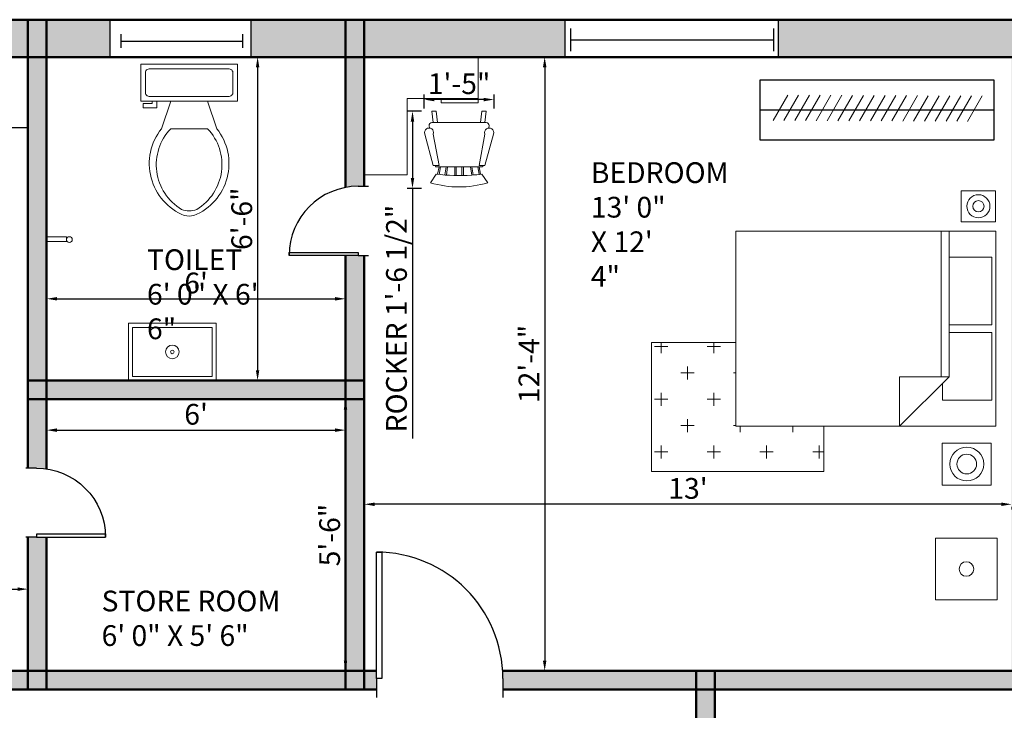
# Model space of a CAD drawing. Units: millimetres. Extents: x 3107 to 3757, y 777 to 1464.
# Tile 6 of 7: x 3301 to 3539, y 1284 to 1450. Entities that reach past the tile are written whole.
import ezdxf

# ---------------------------------------------------------------- set-up
doc = ezdxf.new("R2010")
doc.units = ezdxf.units.MM
for name, color, linetype, lineweight in [('A-ANNO-DIMS', 50, 'Continuous', 18), ('A-AREA-IDEN', 160, 'Continuous', 18), ('A-FLOR-CASE', 140, 'Continuous', 25), ('A-FLOR-CASE-PATT', 140, 'Continuous', 13), ('A-FLOR-FIXT', 140, 'Continuous', 18), ('A-FURN-PATT', 140, 'Continuous', 13), ('A-WALL-PATT', 80, 'Continuous', 13), ('doors', 10, 'Continuous', 25), ('furniture', 140, 'Continuous', 18), ('walls', 80, 'Continuous', 50), ('windows', 30, 'Continuous', 25)]:
    doc.layers.add(name, color=color, linetype=linetype, lineweight=lineweight)
doc.styles.get("Standard").update_dxf_attribs({"font": 'arial.ttf'})
doc.dimstyles.new('ISO-25', dxfattribs={"dimtxt": 5, "dimasz": 2.5, "dimexe": 1.25, "dimexo": 0.625, "dimtad": 1, "dimdec": 0, "dimlunit": 3, "dimtxsty": 'Standard', "dimcen": 2.5, "dimadec": 0, "dimazin": 0, "dimtfac": 1, "dimtdec": 0, "dimtmove": 0, "dimatfit": 3, "dimfxl": 1, "dimarcsym": 0})

# ---------------------------------------------------------------- blocks, each defined once
blk = doc.blocks.new('*U2')
for p, q in [((0, 0), (0, -6)), ((40, 0), (40, -6))]:
    blk.add_line(p, q)
blk.add_lwpolyline([(0, 0), (0, 40), (1.75, 40), (1.75, 0)], close=True)
blk.add_arc((0, 0), 40, 0, 90)
blk = doc.blocks.new('*U5')
for p, q in [((0, 4), (0, 0)), ((36, 4), (36, 0)), ((0, 2), (36, 2))]:
    blk.add_line(p, q)
blk = doc.blocks.new('*U4')
for p, q in [((0, 4), (0, 0)), ((36, 4), (36, 0)), ((0, 2), (36, 2))]:
    blk.add_line(p, q)
blk = doc.blocks.new('Toilet - top')
for p, q in [((9.5, -6), (9.5, -2)), ((-10, -8.5), (-8, -8.5)), ((-10, -9.5), (-10, -8.5)), ((-8, -8.5), (-8, -8)), ((-7, -8), (-7, -9.5)), ((-4, -8), (-6, -14)), ((4, -8), (6, -14)), ((-7, -9.5), (-10, -9.5)), ((4, -14), (-4, -14))]:
    blk.add_line(p, q)
blk.add_lwpolyline([(10.5, -8), (10.5, 0), (-10.5, 0), (-10.5, -8)], close=True)
for points in [[(-9.5, -2), (-9.5, -6)], [(8.5, -1), (-8.5, -1)], [(-8.5, -7), (8.5, -7)]]:
    blk.add_lwpolyline(points)
for centre, radius, start, end in [((-8.62, -1.88), 0.884, 81.8699, 188.1301), ((8.62, -1.88), 0.884, 351.8699, 98.1301), ((-8.62, -6.12), 0.884, 171.8699, 278.1301), ((8.62, -6.12), 0.884, 261.8699, 8.1301), ((3.52, -21.58), 12.17, 141.4691, 247.9714), ((4.2, -21.82), 11.33, 136.3677, 238.9468), ((-3.52, -21.58), 12.17, 292.0284, 38.5307), ((-4.2, -21.82), 11.33, 301.053, 43.6321), ((0, -27.88), 4, 245.7318, 294.2682), ((0, -29), 4, 254.8605, 285.1395)]:
    blk.add_arc(centre, radius, start, end)
blk = doc.blocks.new('Chair - Rocking')
for p, q in [((-8, -4.5), (-10, -1.5)), ((8, -4.5), (10, -1.5)), ((-7.5, -4.5), (-7, -7)), ((-6.5, -7), (-7.02225, -4.43)), ((-4.5, -7), (-4.96674, -4.19951)), ((-4, -7), (-4.40532, -4.16272)), ((-1.5, -4.05012), (-1.5, -7)), ((-1, -7), (-1, -4.05012)), ((1, -7), (1, -4.04655)), ((1.5, -4.05012), (1.5, -7)), ((4, -7), (4.40187, -4.18694)), ((4.5, -7), (4.96761, -4.19437)), ((6.5, -7), (7, -4.4057)), ((7.5, -4.5), (7, -7)), ((-9, -7.5), (-12, -18.49999)), ((-7, -7.5), (-9, -7.5)), ((-9, -18.49999), (-7, -7.5)), ((-8.23428, -6.99939), (-8.3093, -7.47958)), ((-8.23041, -7), (8.23915, -7)), ((7, -7.5), (9, -7.5)), ((9, -18.49999), (7, -7.5)), ((8.31071, -7.48854), (8.23449, -7.00073)), ((9, -7.5), (12, -18.49999)), ((10.5, -21.49999), (10.3575, -20.58798)), ((-10.36644, -20.64523), (-10.5, -21.49999)), ((-9, -22.49999), (-9.5, -26.49999)), ((0, -22.49999), (-9.5, -22.49999)), ((-8, -26.49999), (-7.5, -22.49999)), ((0, -22.49999), (9.5, -22.49999)), ((8, -26.49999), (7.5, -22.49999)), ((9, -22.49999), (9.5, -26.49999)), ((-9.5, -26.49999), (-8, -26.49999)), ((9.5, -26.49999), (8, -26.49999))]:
    blk.add_line(p, q)
for centre, radius, start, end in [((0, -34.08333), 34.08333, 72.93847, 107.0615), ((0, -68.25004), 64.25, 93.92211, 97.15267), ((0, -68.25004), 64.25, 82.84733, 93.92211), ((-10.5, -18.99999), 1.58114, 161.5651, 18.43495), ((10.5, -18.99999), 1.58114, 161.5651, 18.43495), ((-9.5, -21.49999), 1, 180, 270), ((9.5, -21.49999), 1, 270, 0)]:
    blk.add_arc(centre, radius, start, end)
blk = doc.blocks.new('Bed - Queen')
for p, q in [((0, -80.00003), (0, 0)), ((0, 0), (59.99999, 0)), ((59.99999, 0), (59.99999, -80.00003)), ((7.99999, -1.2), (28.79998, -1.2)), ((7.99999, -14.4), (7.99999, -1.2)), ((28.79998, -1.2), (28.79998, -14.4)), ((31.19999, -1.2), (51.99999, -1.2)), ((31.19999, -14.4), (31.19999, -1.2)), ((51.99999, -1.2), (51.99999, -16.4)), ((0, -14.4), (44.8, -14.4)), ((59.99999, -29.6), (44.8, -14.4)), ((44.8, -14.4), (44.8, -29.6)), ((44.8, -16.8), (0, -16.8)), ((51.99999, -16.4), (46.79936, -16.4)), ((44.8, -29.6), (59.99999, -29.6)), ((59.99999, -80.00003), (0, -80.00003))]:
    blk.add_line(p, q)
blk = doc.blocks.new('*D17')
at = {"layer": 'A-ANNO-DIMS', "color": 0, "lineweight": -2, "transparency": 16777216}
for p, q in [((3119.47, 1311.37), (3119.47, 1314.39)), ((3121.97, 1313.14), (3300.97, 1313.14)), ((3303.47, 1313.51), (3303.47, 1311.89))]:
    blk.add_line(p, q, dxfattribs=at)
at = {"layer": 'A-ANNO-DIMS', "color": 0, "transparency": 16777216}
for points in [[(3121.97, 1313.56), (3121.97, 1312.72), (3119.47, 1313.14)], [(3300.97, 1313.56), (3300.97, 1312.72), (3303.47, 1313.14)]]:
    blk.add_solid(points, dxfattribs=at)
at = {"layer": 'Defpoints', "color": 0, "transparency": 16777216}
for p in [(3303.47, 1314.14), (3303.47, 1313.14), (3119.47, 1310.75)]:
    blk.add_point(p, dxfattribs=at)
at = {"layer": 'A-ANNO-DIMS', "color": 0, "transparency": 16777216, "insert": (3211.47, 1316.32), "char_height": 5, "attachment_point": 5}
blk.add_mtext('15\'-4"', dxfattribs=at)
blk = doc.blocks.new('*D18')
at = {"layer": 'A-ANNO-DIMS', "color": 0, "lineweight": -2, "transparency": 16777216}
for p, q in [((3358.24, 1441.43), (3357.54, 1441.43)), ((3358.79, 1438.93), (3358.79, 1365.93)), ((3358.24, 1363.43), (3357.54, 1363.43))]:
    blk.add_line(p, q, dxfattribs=at)
at = {"layer": 'A-ANNO-DIMS', "color": 0, "transparency": 16777216}
for points in [[(3358.38, 1438.93), (3359.21, 1438.93), (3358.79, 1441.43)], [(3358.38, 1365.93), (3359.21, 1365.93), (3358.79, 1363.43)]]:
    blk.add_solid(points, dxfattribs=at)
at = {"layer": 'Defpoints', "color": 0, "transparency": 16777216}
for p in [(3358.87, 1441.43), (3358.79, 1363.43), (3358.87, 1363.43)]:
    blk.add_point(p, dxfattribs=at)
at = {"layer": 'A-ANNO-DIMS', "color": 0, "transparency": 16777216, "insert": (3355.62, 1402.43), "char_height": 5, "attachment_point": 5, "rotation": 90}
blk.add_mtext('6\'-6"', dxfattribs=at)
blk = doc.blocks.new('*D19')
at = {"layer": 'A-ANNO-DIMS', "color": 0, "lineweight": -2, "transparency": 16777216}
for p, q in [((3307.97, 1383.76), (3307.97, 1384.39)), ((3310.47, 1383.14), (3377.47, 1383.14)), ((3379.97, 1383.76), (3379.97, 1384.39))]:
    blk.add_line(p, q, dxfattribs=at)
at = {"layer": 'A-ANNO-DIMS', "color": 0, "transparency": 16777216}
for points in [[(3310.47, 1383.55), (3310.47, 1382.72), (3307.97, 1383.14)], [(3377.47, 1383.55), (3377.47, 1382.72), (3379.97, 1383.14)]]:
    blk.add_solid(points, dxfattribs=at)
at = {"layer": 'Defpoints', "color": 0, "transparency": 16777216}
for p in [(3307.97, 1383.14), (3379.97, 1383.14), (3379.97, 1383.14)]:
    blk.add_point(p, dxfattribs=at)
at = {"layer": 'A-ANNO-DIMS', "color": 0, "transparency": 16777216, "insert": (3343.97, 1386.31), "char_height": 5, "attachment_point": 5}
blk.add_mtext("6'", dxfattribs=at)
blk = doc.blocks.new('*D20')
at = {"layer": 'A-ANNO-DIMS', "color": 0, "lineweight": -2, "transparency": 16777216}
for p, q in [((3384.47, 1334.22), (3384.47, 1334.85)), ((3537.97, 1333.6), (3386.97, 1333.6)), ((3540.47, 1332.97), (3540.47, 1332.35))]:
    blk.add_line(p, q, dxfattribs=at)
at = {"layer": 'A-ANNO-DIMS', "color": 0, "transparency": 16777216}
for points in [[(3386.97, 1334.01), (3386.97, 1333.18), (3384.47, 1333.6)], [(3537.97, 1334.01), (3537.97, 1333.18), (3540.47, 1333.6)]]:
    blk.add_solid(points, dxfattribs=at)
at = {"layer": 'Defpoints', "color": 0, "transparency": 16777216}
for p in [(3384.47, 1333.6), (3384.47, 1333.6), (3540.47, 1333.6)]:
    blk.add_point(p, dxfattribs=at)
at = {"layer": 'A-ANNO-DIMS', "color": 0, "transparency": 16777216, "insert": (3462.47, 1336.78), "char_height": 5, "attachment_point": 5}
blk.add_mtext("13'", dxfattribs=at)
blk = doc.blocks.new('*D21')
at = {"layer": 'A-ANNO-DIMS', "color": 0, "lineweight": -2, "transparency": 16777216}
for p, q in [((3427.43, 1441.43), (3426.7, 1441.43)), ((3427.95, 1438.93), (3427.95, 1295.93)), ((3427.43, 1293.43), (3426.7, 1293.43))]:
    blk.add_line(p, q, dxfattribs=at)
at = {"layer": 'A-ANNO-DIMS', "color": 0, "transparency": 16777216}
for points in [[(3427.53, 1438.93), (3428.37, 1438.93), (3427.95, 1441.43)], [(3427.53, 1295.93), (3428.37, 1295.93), (3427.95, 1293.43)]]:
    blk.add_solid(points, dxfattribs=at)
at = {"layer": 'Defpoints', "color": 0, "transparency": 16777216}
for p in [(3428.06, 1441.43), (3427.95, 1293.43), (3428.06, 1293.43)]:
    blk.add_point(p, dxfattribs=at)
at = {"layer": 'A-ANNO-DIMS', "color": 0, "transparency": 16777216, "insert": (3424.82, 1367.43), "char_height": 5, "attachment_point": 5, "rotation": 90}
blk.add_mtext('12\'-4"', dxfattribs=at)
blk = doc.blocks.new('*D30')
at = {"layer": 'A-ANNO-DIMS', "color": 0, "lineweight": -2, "transparency": 16777216}
for p, q in [((3376.06, 1358.93), (3381.22, 1358.93)), ((3379.97, 1356.43), (3379.97, 1295.93)), ((3376.06, 1293.43), (3381.22, 1293.43))]:
    blk.add_line(p, q, dxfattribs=at)
at = {"layer": 'A-ANNO-DIMS', "color": 0, "transparency": 16777216}
for points in [[(3379.55, 1356.43), (3380.38, 1356.43), (3379.97, 1358.93)], [(3379.55, 1295.93), (3380.38, 1295.93), (3379.97, 1293.43)]]:
    blk.add_solid(points, dxfattribs=at)
at = {"layer": 'Defpoints', "color": 0, "transparency": 16777216}
for p in [(3375.43, 1358.93), (3375.43, 1293.43), (3379.97, 1293.43)]:
    blk.add_point(p, dxfattribs=at)
at = {"layer": 'A-ANNO-DIMS', "color": 0, "transparency": 16777216, "insert": (3376.79, 1326.18), "char_height": 5, "attachment_point": 5, "rotation": 90}
blk.add_mtext('5\'-6"', dxfattribs=at)
blk = doc.blocks.new('*D31')
at = {"layer": 'A-ANNO-DIMS', "color": 0, "lineweight": -2, "transparency": 16777216}
for p, q in [((3307.97, 1354.39), (3307.97, 1350.22)), ((3379.97, 1352.2), (3379.97, 1350.22)), ((3310.47, 1351.47), (3377.47, 1351.47))]:
    blk.add_line(p, q, dxfattribs=at)
at = {"layer": 'A-ANNO-DIMS', "color": 0, "transparency": 16777216}
for points in [[(3310.47, 1351.89), (3310.47, 1351.05), (3307.97, 1351.47)], [(3377.47, 1351.89), (3377.47, 1351.05), (3379.97, 1351.47)]]:
    blk.add_solid(points, dxfattribs=at)
at = {"layer": 'Defpoints', "color": 0, "transparency": 16777216}
for p in [(3307.97, 1355.02), (3379.97, 1352.83), (3379.97, 1351.47)]:
    blk.add_point(p, dxfattribs=at)
at = {"layer": 'A-ANNO-DIMS', "color": 0, "transparency": 16777216, "insert": (3343.97, 1354.65), "char_height": 5, "attachment_point": 5}
blk.add_mtext("6'", dxfattribs=at)
blk = doc.blocks.new('*D67')
at = {"layer": 'A-ANNO-DIMS', "color": 0, "lineweight": -2, "transparency": 16777216}
for p, q in [((3398.27, 1428.37), (3394.86, 1428.37)), ((3396.11, 1425.87), (3396.11, 1412.25)), ((3398.27, 1409.75), (3394.86, 1409.75)), ((3396.11, 1409.75), (3396.11, 1349.49))]:
    blk.add_line(p, q, dxfattribs=at)
at = {"layer": 'A-ANNO-DIMS', "color": 0, "transparency": 16777216}
for points in [[(3395.69, 1425.87), (3396.52, 1425.87), (3396.11, 1428.37)], [(3395.69, 1412.25), (3396.52, 1412.25), (3396.11, 1409.75)]]:
    blk.add_solid(points, dxfattribs=at)
at = {"layer": 'Defpoints', "color": 0, "transparency": 16777216}
for p in [(3398.9, 1428.37), (3396.11, 1409.75), (3398.9, 1409.75)]:
    blk.add_point(p, dxfattribs=at)
at = {"layer": 'A-ANNO-DIMS', "color": 0, "transparency": 16777216, "insert": (3392.89, 1378.37), "char_height": 5, "attachment_point": 5, "rotation": 90}
blk.add_mtext('ROCKER 1\'-6 1/2"', dxfattribs=at)
blk = doc.blocks.new('*D68')
at = {"layer": 'A-ANNO-DIMS', "color": 0, "lineweight": -2, "transparency": 16777216}
for p, q in [((3398.9, 1429), (3398.9, 1432.42)), ((3413.26, 1431.17), (3401.4, 1431.17)), ((3415.76, 1429), (3415.76, 1432.42))]:
    blk.add_line(p, q, dxfattribs=at)
at = {"layer": 'A-ANNO-DIMS', "color": 0, "transparency": 16777216}
for points in [[(3401.4, 1431.58), (3401.4, 1430.75), (3398.9, 1431.17)], [(3413.26, 1431.58), (3413.26, 1430.75), (3415.76, 1431.17)]]:
    blk.add_solid(points, dxfattribs=at)
at = {"layer": 'Defpoints', "color": 0, "transparency": 16777216}
for p in [(3398.9, 1431.17), (3398.9, 1428.37), (3415.76, 1428.37)]:
    blk.add_point(p, dxfattribs=at)
at = {"layer": 'A-ANNO-DIMS', "color": 0, "transparency": 16777216, "insert": (3407.33, 1434.35), "char_height": 5, "attachment_point": 5}
blk.add_mtext('1\'-5"', dxfattribs=at)

msp = doc.modelspace()

# ---------------------------------------------------------------- hatches: boundary and pattern name
at = {"layer": 'A-FLOR-CASE-PATT'}
h = msp.add_hatch(dxfattribs=at)
h.set_pattern_fill('ANSI31', color=256, scale=0.711915, angle=15, style=0)
h.paths.add_polyline_path([(3481.69, 1426.13), (3484.29, 1426.12), (3507.72, 1426.02), (3528.55, 1425.93), (3531.15, 1425.91), (3534.69, 1432.04), (3529.48, 1432.06), (3493.03, 1432.22), (3487.82, 1432.24), (3485.22, 1432.25)])
at = {"layer": 'A-FURN-PATT'}
h = msp.add_hatch(dxfattribs=at)
h.set_pattern_fill('CROSS', color=256)
h.paths.add_polyline_path([(3473.96, 1372.57), (3453.7, 1372.57), (3453.7, 1341.53), (3495.2, 1341.53), (3495.2, 1352.43), (3473.96, 1352.43)])
at = {"layer": 'A-WALL-PATT'}
h = msp.add_hatch(color=256, dxfattribs=at)
h.dxf.hatch_style = 1
h.paths.add_polyline_path([(3119.47, 1087.39), (3110.47, 1087.39), (3110.47, 1027.93), (3119.47, 1027.93)])
h.paths.add_polyline_path([(3119.47, 1027.93), (3110.47, 1027.93), (3110.47, 1023.43), (3119.47, 1023.43)])
h.paths.add_polyline_path([(3267.47, 1027.93), (3119.47, 1027.93), (3119.47, 1023.43), (3267.47, 1023.43)])
h.paths.add_polyline_path([(3119.47, 1023.43), (3110.47, 1023.43), (3110.47, 979.44), (3119.47, 979.44)])
h.paths.add_polyline_path([(3299.97, 1179.93), (3295.47, 1179.93), (3295.47, 1027.93), (3299.97, 1027.93)])
h.paths.add_polyline_path([(3295.47, 1027.93), (3271.97, 1027.93), (3271.97, 1023.43), (3295.47, 1023.43)])
h.paths.add_polyline_path([(3271.97, 1027.93), (3267.47, 1027.93), (3267.47, 1023.43), (3271.97, 1023.43)])
h.paths.add_polyline_path([(3299.97, 1027.93), (3295.47, 1027.93), (3295.47, 1023.43), (3299.97, 1023.43)])
h.paths.add_polyline_path([(3299.97, 1184.43), (3295.47, 1184.43), (3295.47, 1179.93), (3299.97, 1179.93)])
h.paths.add_polyline_path([(3295.47, 1184.43), (3288.38, 1184.43), (3288.38, 1182.47), (3288.38, 1179.93), (3295.47, 1179.93)])
h.paths.add_polyline_path([(3352.47, 1179.93), (3347.97, 1179.93), (3347.97, 1027.93), (3352.47, 1027.93)])
h.paths.add_polyline_path([(3352.47, 1184.43), (3347.97, 1184.43), (3347.97, 1179.93), (3352.47, 1179.93)])
h.paths.add_polyline_path([(3464.47, 1184.43), (3352.47, 1184.43), (3352.47, 1179.93), (3464.47, 1179.93)])
h.paths.add_polyline_path([(3468.97, 1288.93), (3464.47, 1288.93), (3464.47, 1184.43), (3468.97, 1184.43)])
h.paths.add_polyline_path([(3468.97, 1184.43), (3464.47, 1184.43), (3464.47, 1179.93), (3468.97, 1179.93)])
h.paths.add_polyline_path([(3195.97, 1248.43), (3191.47, 1248.43), (3191.47, 1184.43), (3195.97, 1184.43)])
h.paths.add_polyline_path([(3195.97, 1184.43), (3191.47, 1184.43), (3191.47, 1179.93), (3195.97, 1179.93)])
h.paths.add_polyline_path([(3191.47, 1184.43), (3183.28, 1184.43), (3183.28, 1181.58), (3183.28, 1179.93), (3191.47, 1179.93)])
h.paths.add_polyline_path([(3243.97, 1184.43), (3195.97, 1184.43), (3195.97, 1179.93), (3243.97, 1179.93)])
h.paths.add_polyline_path([(3257.91, 1182.47), (3257.91, 1184.43), (3248.47, 1184.43), (3248.47, 1179.93), (3258.02, 1179.93, -0.020891)])
h.paths.add_polyline_path([(3248.47, 1184.43), (3243.97, 1184.43), (3243.97, 1179.93), (3248.47, 1179.93)])
h.paths.add_polyline_path([(3248.47, 1189.24), (3247.51, 1189.24), (3243.97, 1189.24), (3243.97, 1184.43), (3248.47, 1184.43)])
h.paths.add_polyline_path([(3166.87, 1184.43), (3119.47, 1184.43), (3119.47, 1179.93), (3166.63, 1179.93), (3166.63, 1181.58, -0.042981)])
h.paths.add_polyline_path([(3119.47, 1184.43), (3110.47, 1184.43), (3110.47, 1179.93), (3119.47, 1179.93)])
h.paths.add_polyline_path([(3119.47, 1248.43), (3110.47, 1248.43), (3110.47, 1184.43), (3119.47, 1184.43)])
h.paths.add_polyline_path([(3119.47, 1179.93), (3110.47, 1179.93), (3110.47, 1140.65), (3119.47, 1140.65)])
h.paths.add_polyline_path([(3119.47, 1288.93), (3110.47, 1288.93), (3110.47, 1252.93), (3119.47, 1252.93)])
h.paths.add_polyline_path([(3119.47, 1252.93), (3110.47, 1252.93), (3110.47, 1248.43), (3119.47, 1248.43)])
h.paths.add_polyline_path([(3191.47, 1252.93), (3119.47, 1252.93), (3119.47, 1248.43), (3191.47, 1248.43)])
h.paths.add_polyline_path([(3195.97, 1288.93), (3191.47, 1288.93), (3191.47, 1252.93), (3195.97, 1252.93)])
h.paths.add_polyline_path([(3195.97, 1252.93), (3191.47, 1252.93), (3191.47, 1248.43), (3195.97, 1248.43)])
h.paths.add_polyline_path([(3248.47, 1293.43), (3243.97, 1293.43), (3243.97, 1288.93), (3248.47, 1288.93)])
h.paths.add_polyline_path([(3243.97, 1293.43), (3195.97, 1293.43), (3195.97, 1288.93), (3243.97, 1288.93)])
h.paths.add_polyline_path([(3303.47, 1293.43), (3248.47, 1293.43), (3248.47, 1288.93), (3303.47, 1288.93)])
h.paths.add_polyline_path([(3248.47, 1288.93), (3243.97, 1288.93), (3243.97, 1205.51, -0.053712), (3247.51, 1205.89), (3248.47, 1205.89)])
h.paths.add_polyline_path([(3191.47, 1293.43), (3119.47, 1293.43), (3119.47, 1288.93), (3191.47, 1288.93)])
h.paths.add_polyline_path([(3119.47, 1293.43), (3110.47, 1293.43), (3110.47, 1288.93), (3119.47, 1288.93)])
h.paths.add_polyline_path([(3119.47, 1322.96, -0.065064), (3111.64, 1321.93), (3110.47, 1321.93), (3110.47, 1293.43), (3119.47, 1293.43)])
h.paths.add_polyline_path([(3195.97, 1293.43), (3191.47, 1293.43), (3191.47, 1288.93), (3195.97, 1288.93)])
h.paths.add_polyline_path([(3119.47, 1450.43), (3110.47, 1450.43), (3110.47, 1441.43), (3119.47, 1441.43)])
h.paths.add_polyline_path([(3119.47, 1441.43), (3110.47, 1441.43), (3110.47, 1352.4), (3111.64, 1352.4), (3119.47, 1352.4)])
h.paths.add_polyline_path([(3176.58, 1450.43), (3119.47, 1450.43), (3119.47, 1441.43), (3176.58, 1441.43)])
h.paths.add_polyline_path([(3323.19, 1450.43), (3307.97, 1450.43), (3307.97, 1441.43), (3323.19, 1441.43)])
h.paths.add_polyline_path([(3307.97, 1450.43), (3303.47, 1450.43), (3303.47, 1441.43), (3307.97, 1441.43)])
h.paths.add_polyline_path([(3303.47, 1450.43), (3229.4, 1450.43), (3229.4, 1441.43), (3303.47, 1441.43)])
h.paths.add_polyline_path([(3307.97, 1441.43), (3303.47, 1441.43), (3303.47, 1363.43), (3307.97, 1363.43)])
h.paths.add_polyline_path([(3307.97, 1363.43), (3303.47, 1363.43), (3303.47, 1358.93), (3307.97, 1358.93)])
h.paths.add_polyline_path([(3307.97, 1358.93), (3303.47, 1358.93), (3303.47, 1342.3), (3305.5, 1342.3, -0.037178), (3307.97, 1342.12)])
h.paths.add_polyline_path([(3379.97, 1363.43), (3307.97, 1363.43), (3307.97, 1358.93), (3379.97, 1358.93)])
h.paths.add_polyline_path([(3384.47, 1393.61), (3383.04, 1393.61), (3379.97, 1393.61), (3379.97, 1363.43), (3384.47, 1363.43)])
h.paths.add_polyline_path([(3384.47, 1363.43), (3379.97, 1363.43), (3379.97, 1358.93), (3384.47, 1358.93)])
h.paths.add_polyline_path([(3384.47, 1358.93), (3379.97, 1358.93), (3379.97, 1293.43), (3384.47, 1293.43)])
h.paths.add_polyline_path([(3384.47, 1441.43), (3379.97, 1441.43), (3379.97, 1409.98, -0.046389), (3383.04, 1410.27), (3384.47, 1410.27)])
h.paths.add_polyline_path([(3384.47, 1450.43), (3379.97, 1450.43), (3379.97, 1441.43), (3384.47, 1441.43)])
h.paths.add_polyline_path([(3379.97, 1450.43), (3357.18, 1450.43), (3357.18, 1441.43), (3379.97, 1441.43)])
h.paths.add_polyline_path([(3432.79, 1450.43), (3384.47, 1450.43), (3384.47, 1441.43), (3432.79, 1441.43)])
h.paths.add_polyline_path([(3540.47, 1450.43), (3484.18, 1450.43), (3484.18, 1441.43), (3540.47, 1441.43)])
h.paths.add_polyline_path([(3544.97, 1450.43), (3540.47, 1450.43), (3540.47, 1441.43), (3544.97, 1441.43)])
h.paths.add_polyline_path([(3544.97, 1441.43), (3540.47, 1441.43), (3540.47, 1293.43), (3544.97, 1293.43)])
h.paths.add_polyline_path([(3590.83, 1450.43), (3544.97, 1450.43), (3544.97, 1441.43), (3590.83, 1441.43)])
h.paths.add_polyline_path([(3712.97, 1450.43), (3645.62, 1450.43), (3645.62, 1441.43), (3712.97, 1441.43)])
h.paths.add_polyline_path([(3721.97, 1441.43), (3712.97, 1441.43), (3712.97, 1288.93), (3712.97, 1184.43), (3721.97, 1184.43), (3721.97, 1288.93)])
h.paths.add_polyline_path([(3721.97, 1450.43), (3712.97, 1450.43), (3712.97, 1441.43), (3721.97, 1441.43)])
h.paths.add_polyline_path([(3712.97, 1184.43), (3658.24, 1184.43), (3658.24, 1183.15), (3658.24, 1179.93), (3712.97, 1179.93)])
h.paths.add_polyline_path([(3721.97, 1184.43), (3712.97, 1184.43), (3712.97, 1179.93), (3721.97, 1179.93)])
h.paths.add_polyline_path([(3597.32, 1183.15), (3597.32, 1184.43), (3544.97, 1184.43), (3544.97, 1179.93), (3597.32, 1179.93)])
h.paths.add_polyline_path([(3544.97, 1184.43), (3540.47, 1184.43), (3540.47, 1179.93), (3544.97, 1179.93)])
h.paths.add_polyline_path([(3544.97, 1179.93), (3540.47, 1179.93), (3540.47, 1143.69), (3543.65, 1143.69), (3544.97, 1143.69)])
h.paths.add_polyline_path([(3721.97, 1179.93), (3712.97, 1179.93), (3712.97, 1006.22), (3712.97, 871.43), (3721.97, 871.43), (3721.97, 1006.22)])
h.paths.add_polyline_path([(3468.97, 1293.43), (3464.47, 1293.43), (3464.47, 1288.93), (3468.97, 1288.93)])
h.paths.add_polyline_path([(3540.47, 1293.43), (3468.97, 1293.43), (3468.97, 1288.93), (3540.47, 1288.93)])
h.paths.add_polyline_path([(3544.97, 1293.43), (3540.47, 1293.43), (3540.47, 1288.93), (3544.97, 1288.93)])
h.paths.add_polyline_path([(3464.47, 1293.43), (3417.83, 1293.43, -0.015057), (3417.88, 1291.6), (3417.88, 1288.93), (3464.47, 1288.93)])
h.paths.add_polyline_path([(3379.97, 1293.43), (3307.97, 1293.43), (3307.97, 1288.93), (3379.97, 1288.93)])
h.paths.add_polyline_path([(3307.97, 1325.65), (3305.5, 1325.65), (3303.47, 1325.65), (3303.47, 1293.43), (3307.97, 1293.43)])
h.paths.add_polyline_path([(3307.97, 1293.43), (3303.47, 1293.43), (3303.47, 1288.93), (3307.97, 1288.93)])
h.paths.add_polyline_path([(3384.47, 1293.43), (3379.97, 1293.43), (3379.97, 1288.93), (3384.47, 1288.93)])
h.paths.add_polyline_path([(3387.42, 1291.6), (3387.42, 1293.43), (3384.47, 1293.43), (3384.47, 1288.93), (3387.42, 1288.93)])
h.paths.add_polyline_path([(3119.47, 927.28), (3110.47, 927.28), (3110.47, 871.43), (3119.47, 871.43)])
h.paths.add_polyline_path([(3119.47, 871.43), (3110.47, 871.43), (3110.47, 862.43), (3119.47, 862.43)])
h.paths.add_polyline_path([(3267.47, 871.43), (3119.47, 871.43), (3119.47, 862.43), (3267.47, 862.43)])
h.paths.add_polyline_path([(3271.97, 971.43), (3267.47, 971.43), (3267.47, 871.43), (3271.97, 871.43)])
h.paths.add_polyline_path([(3271.97, 871.43), (3267.47, 871.43), (3267.47, 862.43), (3271.97, 862.43)])
h.paths.add_polyline_path([(3287.13, 871.43), (3271.97, 871.43), (3271.97, 862.43), (3287.13, 862.43)])
h.paths.add_polyline_path([(3347.97, 871.43), (3318.96, 871.43), (3318.96, 862.43), (3347.97, 862.43)])
h.paths.add_polyline_path([(3352.47, 971.43), (3347.97, 971.43), (3347.97, 871.43), (3352.47, 871.43)])
h.paths.add_polyline_path([(3352.47, 871.43), (3347.97, 871.43), (3347.97, 862.43), (3352.47, 862.43)])
h.paths.add_polyline_path([(3375.96, 871.43), (3352.47, 871.43), (3352.47, 862.43), (3375.96, 862.43)])
h.paths.add_polyline_path([(3352.47, 975.93), (3347.97, 975.93), (3347.97, 971.43), (3352.47, 971.43)])
h.paths.add_polyline_path([(3352.47, 986.27, -0.01722), (3350.37, 986.2), (3347.97, 986.2), (3347.97, 975.93), (3352.47, 975.93)])
h.paths.add_polyline_path([(3347.97, 975.93), (3292.38, 975.93), (3292.38, 973.47, -0.030785), (3292.25, 971.43), (3347.97, 971.43)])
h.paths.add_polyline_path([(3271.97, 985.98), (3269.95, 985.98), (3267.47, 985.98), (3267.47, 975.93), (3271.97, 975.93)])
h.paths.add_polyline_path([(3271.97, 975.93), (3267.47, 975.93), (3267.47, 971.43), (3271.97, 971.43)])
h.paths.add_polyline_path([(3275.72, 975.93), (3271.97, 975.93), (3271.97, 971.43), (3275.72, 971.43), (3275.72, 973.47)])
h.paths.add_polyline_path([(3271.97, 1023.43), (3267.47, 1023.43), (3267.47, 1016.34, -0.020418), (3269.95, 1016.44), (3271.97, 1016.44)])
h.paths.add_polyline_path([(3352.47, 1023.43), (3347.97, 1023.43), (3347.97, 1016.67), (3350.37, 1016.67), (3352.47, 1016.67)])
h.paths.add_polyline_path([(3352.47, 1027.93), (3347.97, 1027.93), (3347.97, 1023.43), (3352.47, 1023.43)])
h.paths.add_polyline_path([(3476.47, 1027.93), (3352.47, 1027.93), (3352.47, 1023.43), (3476.47, 1023.43)])
h.paths.add_polyline_path([(3540.47, 1027.93), (3480.97, 1027.93), (3480.97, 1023.43), (3540.47, 1023.43)])
h.paths.add_polyline_path([(3480.97, 1027.93), (3476.47, 1027.93), (3476.47, 1023.43), (3480.97, 1023.43)])
h.paths.add_polyline_path([(3480.97, 1023.43), (3476.47, 1023.43), (3476.47, 871.43), (3480.97, 871.43)])
h.paths.add_polyline_path([(3476.47, 871.43), (3429.88, 871.43), (3429.88, 862.43), (3476.47, 862.43)])
h.paths.add_polyline_path([(3480.97, 871.43), (3476.47, 871.43), (3476.47, 862.43), (3480.97, 862.43)])
h.paths.add_polyline_path([(3493.81, 871.43), (3480.97, 871.43), (3480.97, 862.43), (3493.81, 862.43)])
h.paths.add_polyline_path([(3712.97, 871.43), (3525.61, 871.43), (3525.61, 862.43), (3712.97, 862.43)])
h.paths.add_polyline_path([(3721.97, 871.43), (3712.97, 871.43), (3712.97, 862.43), (3721.97, 862.43)])

# ---------------------------------------------------------------- linework, layer by layer
at = {"layer": 'A-FLOR-CASE'}
for p, q in [((3303.47, 1441.43), (3303.47, 1424.33)), ((3479.78, 1428.67), (3536.26, 1428.67)), ((3303.47, 1424.33), (3136.75, 1424.33))]:
    msp.add_line(p, q, dxfattribs=at)
msp.add_lwpolyline([(3536.26, 1435.88), (3479.78, 1435.88), (3479.78, 1421.45), (3536.26, 1421.45)], close=True, dxfattribs=at)
at = {"layer": 'A-FLOR-FIXT'}
msp.add_line((3307.97, 1400.06), (3307.97, 1400.06), dxfattribs=at)
for points in [[(3307.97, 1398.04), (3312.77, 1398.04), (3312.77, 1396.98), (3307.97, 1396.98)], [(3327.68, 1377.23), (3348.82, 1377.23), (3348.82, 1363.43), (3327.68, 1363.43)], [(3328.68, 1376.23), (3347.82, 1376.23), (3347.82, 1364.43), (3328.68, 1364.43)]]:
    msp.add_lwpolyline(points, close=True, dxfattribs=at)
for centre, radius in [((3313.45, 1397.41), 0.696), ((3338.25, 1370.33), 1.64), ((3338.25, 1370.33), 0.446)]:
    msp.add_circle(centre, radius, dxfattribs=at)
at = {"layer": 'furniture'}
for p, q in [((3411.91, 1431.41), (3403.03, 1431.41)), ((3411.91, 1431.41), (3403.03, 1431.41)), ((3411.91, 1430.41), (3403.03, 1430.41)), ((3473.96, 1372.57), (3453.7, 1372.57)), ((3453.7, 1372.57), (3453.7, 1341.53)), ((3495.2, 1341.53), (3495.2, 1352.43)), ((3453.7, 1341.53), (3495.2, 1341.53))]:
    msp.add_line(p, q, dxfattribs=at)
for points in [[(3394.8, 1431.41), (3394.8, 1413.02), (3384.47, 1413.02), (3384.47, 1441.43), (3394.8, 1441.43)], [(3384.47, 1431.41), (3384.47, 1441.43), (3411.91, 1441.43), (3411.91, 1431.41), (3394.8, 1431.41)]]:
    msp.add_lwpolyline(points, dxfattribs=at)
for points in [[(3403.03, 1431.41), (3411.91, 1431.41), (3411.91, 1430.37), (3403.03, 1430.37)], [(3536.57, 1401.73), (3528.29, 1401.73), (3528.29, 1409.15), (3536.57, 1409.15)], [(3535.53, 1348.36), (3523.73, 1348.36), (3523.73, 1338.24), (3535.53, 1338.24)], [(3522.11, 1325.42), (3536.98, 1325.42), (3536.98, 1310.56), (3522.11, 1310.56)]]:
    msp.add_lwpolyline(points, close=True, dxfattribs=at)
for centre, radius in [((3532.43, 1405.44), 2.78), ((3532.43, 1405.44), 1.37), ((3529.63, 1343.3), 4.08), ((3529.63, 1343.3), 2.37), ((3529.54, 1317.99), 1.76)]:
    msp.add_circle(centre, radius, dxfattribs=at)
at = {"layer": 'walls'}
for p, q in [((3110.47, 1450.43), (3721.97, 1450.43)), ((3303.47, 1450.43), (3303.47, 1363.43)), ((3307.97, 1450.43), (3307.97, 1363.43)), ((3379.97, 1450.43), (3379.97, 1409.98)), ((3384.47, 1450.43), (3384.47, 1410.27)), ((3110.47, 1441.43), (3721.97, 1441.43)), ((3379.97, 1393.61), (3379.97, 1288.93)), ((3384.47, 1393.61), (3384.47, 1288.93)), ((3303.47, 1386.3), (3303.47, 1342.3)), ((3307.97, 1386.49), (3307.97, 1342.12)), ((3303.47, 1363.43), (3384.47, 1363.43)), ((3303.47, 1358.93), (3384.47, 1358.93)), ((3303.47, 1325.65), (3303.47, 1288.93)), ((3307.97, 1325.65), (3307.97, 1288.93)), ((3110.47, 1293.43), (3384.47, 1293.43)), ((3110.47, 1293.43), (3387.42, 1293.43)), ((3417.83, 1293.43), (3544.97, 1293.43)), ((3464.47, 1293.43), (3464.47, 1179.93)), ((3468.97, 1293.43), (3468.97, 1179.93)), ((3110.47, 1288.93), (3384.47, 1288.93)), ((3110.47, 1288.93), (3387.42, 1288.93)), ((3417.88, 1288.93), (3544.97, 1288.93))]:
    msp.add_line(p, q, dxfattribs=at)
at = {"layer": 'windows'}
for p, q in [((3323.19, 1450.43), (3323.19, 1441.43)), ((3357.18, 1450.43), (3357.18, 1441.43)), ((3432.79, 1450.43), (3432.79, 1441.43)), ((3484.18, 1450.43), (3484.18, 1441.43))]:
    msp.add_line(p, q, dxfattribs=at)

# ---------------------------------------------------------------- block references
at = {"layer": 'A-FLOR-FIXT', "xscale": 1.109949414103811, "yscale": 1.109949414103811, "zscale": 1.109949414103811}
msp.add_blockref('Toilet - top', (3342.3, 1439.69), dxfattribs=at)
at = {"layer": 'doors', "yscale": 0.4163085604342208, "zscale": 0.4163085604342208}
for p, xscale, rotation in [((3383.04, 1393.61), 0.4163085604342208, 90.00000000000003), ((3305.5, 1325.65), -0.4163085604342208, 270)]:
    msp.add_blockref('*U2', p, dxfattribs=dict(at, xscale=xscale, rotation=rotation))
at = {"layer": 'doors', "xscale": 0.7615706373352984, "yscale": 0.7615706373352984, "zscale": 0.7615706373352984}
msp.add_blockref('*U2', (3387.42, 1291.6), dxfattribs=at)
at = {"layer": 'furniture'}
for name, p, xscale, yscale, zscale, rotation in [('Chair - Rocking', (3407.33, 1410.09), 0.6898552629490491, 0.6898552629490491, 0.6898552629490491, 180), ('Bed - Queen', (3536.64, 1399.44), 0.7835133119924312, 0.7835133119924312, 0.7835133119924312, 270.0000000000084)]:
    msp.add_blockref(name, p, dxfattribs=dict(at, xscale=xscale, yscale=yscale, zscale=zscale, rotation=rotation))
at = {"layer": 'windows'}
for name, p, xscale, yscale, zscale in [('*U5', (3325.81, 1443.65), 0.8150463067894532, 0.8150463067894532, 0.8150463067894532), ('*U4', (3434.19, 1442.86), 1.357941570966636, 1.357941570966636, 1.357941570966636)]:
    msp.add_blockref(name, p, dxfattribs=dict(at, xscale=xscale, yscale=yscale, zscale=zscale))

# ---------------------------------------------------------------- texts
at = {"layer": 'A-AREA-IDEN', "char_height": 5, "attachment_point": 1}
for s, width, insert in [('BEDROOM \\P13\' 0" X 12\' 4"', 22.5448, (3439.07, 1416.05)), ('TOILET \\P6\' 0" X 6\' 6"', 31.6268, (3332.15, 1395.07)), ('STORE ROOM \\P6\' 0" X 5\' 6"', 55.2686, (3321.21, 1312.78))]:
    msp.add_mtext_dynamic_manual_height_columns(s, width=width, gutter_width=12.5, heights=[0], dxfattribs=dict(at, insert=insert))

# ---------------------------------------------------------------- dimensions: what is measured, and where the dimension line sits
at = {"layer": 'A-ANNO-DIMS'}
for base, p1, p2, angle, override, picture, middle in [((3358.79, 1363.43), (3358.87, 1441.43), (3358.87, 1363.43), 90, {"dimclrd": 0, "dimclre": 0, "dimclrt": 0}, '*D18', (3355.62, 1402.43)), ((3427.95, 1293.43), (3428.06, 1441.43), (3428.06, 1293.43), 90, {"dimclrd": 0, "dimclre": 0, "dimclrt": 0}, '*D21', (3424.82, 1367.43)), ((3398.9, 1431.17), (3415.76, 1428.37), (3398.9, 1428.37), 180, {"dimdec": 1, "dimlfac": 1, "dimrnd": 0, "dimzin": 1, "dimdsep": 46, "dimlunit": 4, "dimfrac": 2}, '*D68', (3407.33, 1434.35)), ((3379.96513133, 1293.42857409), (3375.43350517, 1358.92857409), (3375.43350517, 1293.42857409), 90, {"dimclrd": 0, "dimclre": 0, "dimclrt": 0}, '*D30', (3376.78726639, 1326.17857409))]:
    dim = msp.add_linear_dim(base=base, p1=p1, p2=p2, angle=angle, dimstyle='ISO-25', override=override, dxfattribs=at)
    dim.commit()
    dim.dimension.update_dxf_attribs({"geometry": picture, "text_midpoint": middle})
dim = msp.add_linear_dim(base=(3396.11, 1409.75), p1=(3398.9, 1428.37), p2=(3398.9, 1409.75), angle=270, text='ROCKER <>', dimstyle='ISO-25', override={"dimdec": 1, "dimlfac": 1, "dimrnd": 0, "dimzin": 1, "dimdsep": 46, "dimlunit": 4, "dimfrac": 2}, dxfattribs=at)
dim.commit()
dim.dimension.update_dxf_attribs({"geometry": '*D67', "text_midpoint": (3392.89, 1378.37)})
for base, p1, p2, picture, middle in [((3379.97, 1383.14), (3307.97, 1383.14), (3379.97, 1383.14), '*D19', (3343.97, 1386.31)), ((3379.97, 1351.47), (3307.97, 1355.02), (3379.97, 1352.83), '*D31', (3343.97, 1354.65)), ((3384.47, 1333.6), (3540.47, 1333.6), (3384.47, 1333.6), '*D20', (3462.47, 1336.78)), ((3303.47, 1313.14), (3119.47, 1310.75), (3303.47, 1314.14), '*D17', (3211.47, 1316.32))]:
    dim = msp.add_linear_dim(base=base, p1=p1, p2=p2, dimstyle='ISO-25', override={"dimclrd": 0, "dimclre": 0, "dimclrt": 0}, dxfattribs=at)
    dim.commit()
    dim.dimension.update_dxf_attribs({"geometry": picture, "text_midpoint": middle})

doc.saveas('drawing.dxf')
